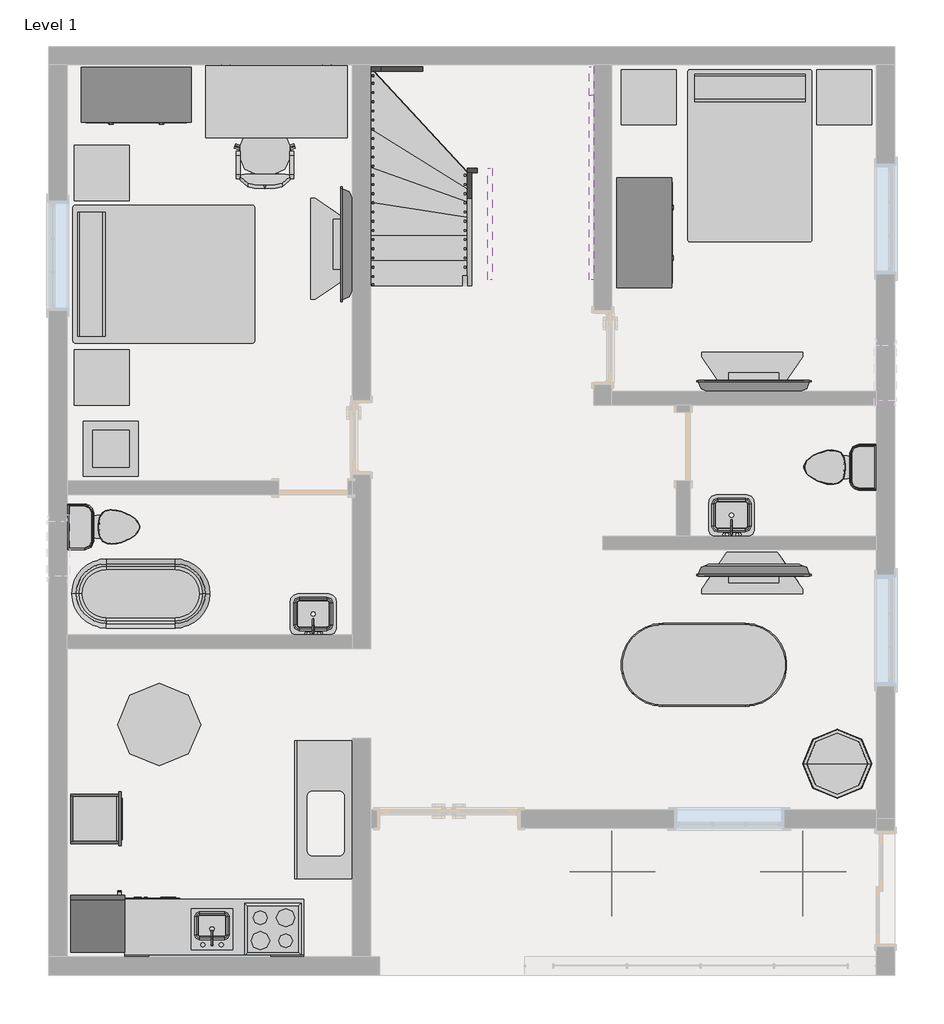
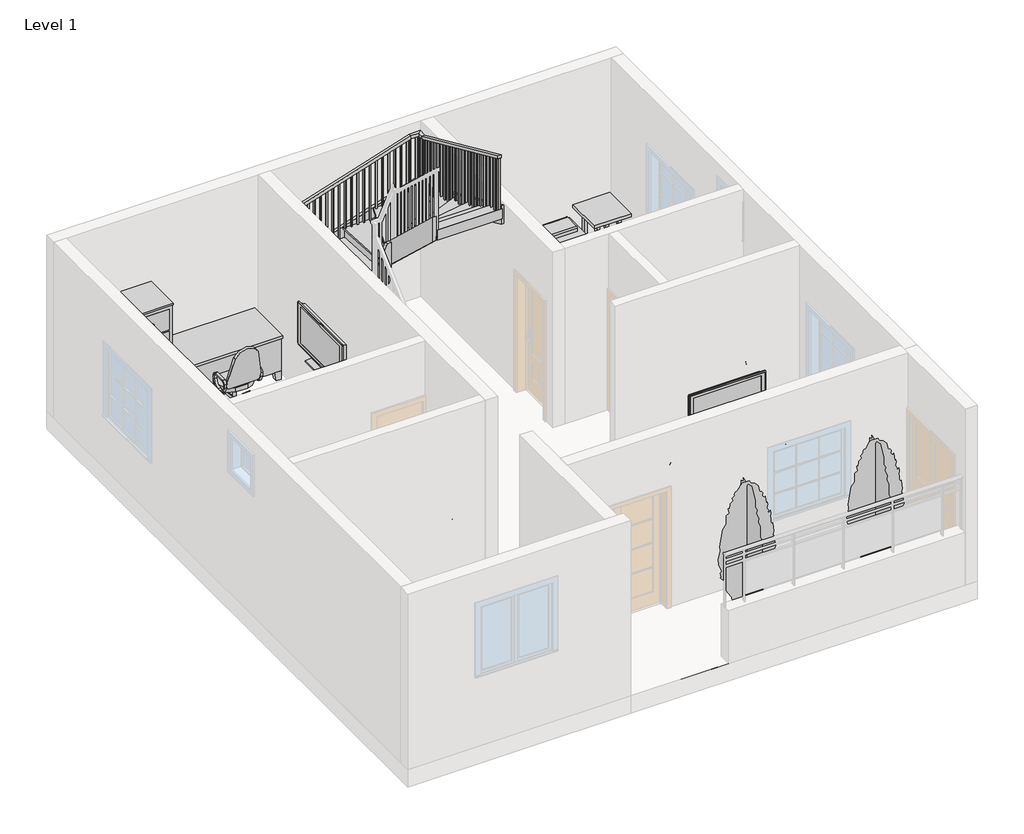
# One storey, part 2 of 2: 22 furniture elements, 8 members, 6 flow terminals, 6 proxies, 2 geographic elements, 1 railing, 1 stair flight.
"""IFC4 building model written with IfcOpenShell, lengths in millimetres."""

from ifc_helpers import new_model, si_unit, frame, origin, place, context, project, spatial, polyline, outline, extrude, faceted_brep, triangles, transform, mapped, element, save
from components import proxy_a6faaae8, proxy_45b28599, kitchenette_medium_kitchenette_medium_844211aa, proxy_8b8c2dc4, proxy_c523a7b7, flow_terminal_871c2e40, flow_terminal_62a433f7, toilet_domestic_3d_toilet_domestic_3d_f7549cf7, toilet_domestic_3d_toilet_domestic_3d_183bbd19, flow_terminal_b374fae2, furniture_0253826f, furniture_e1791683, chair_executive_chair_executive_8d69e98c, furniture_c6510c7c, furniture_6430aa70, furniture_072f6425, furniture_9fa109b2, furniture_fdf74506, tv_stand_tv_stand_6ce107e5, furniture_b5c51a22, furniture_2c34a4f9, furniture_905aceb5, furniture_5bc9ed15, furniture_ebfaaaa6, rpc_tree_conifer_chinese_juniper_7_1b9786cd, stair_flight_3064df67

model = new_model("IFC4")

# Units and contexts
model_context = context("Model", 3, world=origin())
ifc_project = project(units=[si_unit("LENGTHUNIT", "METRE", prefix="MILLI")], contexts=[model_context])

# Site, building, storey
site = spatial("IfcSite", under=ifc_project)
building = spatial("IfcBuilding", under=site)
storey = spatial("IfcBuildingStorey", under=building, Name="Level 1", Elevation=0.0)

# Proxies
placement = place(None, origin())
element("IfcBuildingElementProxy", 1, Name="Building Element Proxy", at=placement, inside=storey, context=model_context, shape_type="Tessellation", body=[
    triangles([(-8321.547876, 2776.9674156, 0.0), (-8317.1533768, 1400.6475002, 0.0), (-8215.9921097, 1395.5161274, 0.0), (-8214.5265015, 1174.0855299, 0.0), (-6665.8942841, 1174.0855299, 0.0), (-6657.047731, 1395.5938843, 0.0), (-6691.0613525, 2780.6355057, 0.0), (-2754.0612556, 2761.5855057, 0.0), (-2754.0612556, 1377.2855541, 0.0)], [[3, 4, 5], [4, 3, 2], [1, 2, 3], [3, 7, 1], [5, 9, 6], [7, 6, 8], [7, 3, 6], [8, 6, 9], [6, 3, 5]], closed=False),
])
proxy_shape = proxy_a6faaae8(model_context)
element("IfcBuildingElementProxy", 2, Name="Cook Top-4 Unit2 : 22\" x 20\"", ObjectType="Cook Top-4 Unit2 : 22\" x 20\"", at=placement, inside=storey, context=model_context, shape_type="MappedRepresentation", body=[
    mapped(proxy_shape, transform((-9421.5611447, 1682.085558, 0.0), x_axis=(-1.0000000000000004, 0.0, 0.0), y_axis=(0.0, -1.0000000000000004, 0.0), z_axis=(0.0, 0.0, 1.0))),
])
proxy_2_shape = proxy_45b28599(model_context)
element("IfcBuildingElementProxy", 3, Name="Dishwasher : 24\" x 24\" x 34\"", ObjectType="Dishwasher : 24\" x 24\" x 34\"", at=placement, inside=storey, context=model_context, shape_type="MappedRepresentation", body=[
    mapped(proxy_2_shape, transform((-10372.7436762, 1973.9351228, 0.0), x_axis=(-1.0000000000000004, 0.0, 0.0), y_axis=(0.0, -1.0000000000000004, 0.0), z_axis=(0.0, 0.0, 1.0))),
])
kitchenette_medium_kitchenette_medium_shape = kitchenette_medium_kitchenette_medium_844211aa(model_context)
element("IfcBuildingElementProxy", 4, Name="Kitchenette - Medium : Kitchenette - Medium", ObjectType="Kitchenette - Medium : Kitchenette - Medium", at=placement, inside=storey, context=model_context, shape_type="MappedRepresentation", body=[
    mapped(kitchenette_medium_kitchenette_medium_shape, transform((-9745.7234398, 1377.285558, 0.0), x_axis=(-1.0000000000000004, 0.0, 0.0), y_axis=(0.0, -1.0000000000000004, 0.0), z_axis=(0.0, 0.0, 1.0))),
])
proxy_3_shape = proxy_8b8c2dc4(model_context)
element("IfcBuildingElementProxy", 5, Name="Oven Double-Built-in : 21 1/2\" x 39 1/4\" x 21\"", ObjectType="Oven Double-Built-in : 21 1/2\" x 39 1/4\" x 21\"", at=placement, inside=storey, context=model_context, shape_type="MappedRepresentation", body=[
    mapped(proxy_3_shape, transform((-11248.9952858, 2936.4604853, 0.0), x_axis=(0.0, 1.0000000000000002, 0.0), y_axis=(-1.0000000000000002, 0.0, 0.0), z_axis=(0.0, 0.0, 1.0))),
])
proxy_4_shape = proxy_c523a7b7(model_context)
element("IfcBuildingElementProxy", 6, Name="Refrigerator : 24\" x 25\" LH", ObjectType="Refrigerator : 24\" x 25\" LH", at=placement, inside=storey, context=model_context, shape_type="MappedRepresentation", body=[
    mapped(proxy_4_shape, transform((-11358.3111447, 1727.7345295, 0.0), x_axis=(-1.0000000000000004, 0.0, 0.0), y_axis=(0.0, -1.0000000000000004, 0.0), z_axis=(0.0, 0.0, 1.0))),
])

# Flow terminals
flow_terminal_shape = flow_terminal_871c2e40(model_context)
element("IfcFlowTerminal", 7, ObjectType="Sink Kitchen-Island : 18\" x 18\"", at=placement, inside=storey, context=model_context, shape_type="MappedRepresentation", body=[
    mapped(flow_terminal_shape, transform((-10078.9719042, 1684.4309591, -14.4), x_axis=(-1.0000000000000004, 0.0, 0.0), y_axis=(0.0, -1.0000000000000004, 0.0), z_axis=(0.0, 0.0, 1.0))),
])
flow_terminal_2_shape = flow_terminal_62a433f7(model_context)
element("IfcFlowTerminal", 8, ObjectType="Sink Vanity-Square : 20\" x 18\"", at=placement, inside=storey, context=model_context, shape_type="MappedRepresentation", body=[
    mapped(flow_terminal_2_shape, transform((-8961.3719042, 5113.4309591, 0.0), x_axis=(-0.9999999999999998, 0.0, 0.0), y_axis=(0.0, -0.9999999999999998, 0.0), z_axis=(0.0, 0.0, 1.0))),
])
element("IfcFlowTerminal", 9, ObjectType="Sink Vanity-Square : 20\" x 18\"", at=placement, inside=storey, context=model_context, shape_type="MappedRepresentation", body=[
    mapped(flow_terminal_2_shape, transform((-4338.5719042, 6205.6309591, 0.0), x_axis=(-1.0, 0.0, 0.0), y_axis=(0.0, -1.0, 0.0), z_axis=(0.0, 0.0, 1.0))),
])
toilet_domestic_3d_toilet_domestic_3d_shape = toilet_domestic_3d_toilet_domestic_3d_f7549cf7(model_context)
toilet_domestic_3d_toilet_domestic_3d_2_shape = toilet_domestic_3d_toilet_domestic_3d_183bbd19(model_context)
element("IfcFlowTerminal", 10, ObjectType="Toilet-Domestic-3D : Toilet-Domestic-3D", at=placement, inside=storey, context=model_context, shape_type="MappedRepresentation", body=[
    mapped(toilet_domestic_3d_toilet_domestic_3d_shape, transform((-11200.1651174, 6127.085558, 0.0), x_axis=(0.0, 1.0000000000000002, 0.0), y_axis=(-1.0000000000000002, 0.0, 0.0), z_axis=(0.0, 0.0, 1.0))),
    mapped(toilet_domestic_3d_toilet_domestic_3d_2_shape, transform((-11200.1651174, 6127.085558, 0.0), x_axis=(0.0, 1.0000000000000002, 0.0), y_axis=(-1.0000000000000002, 0.0, 0.0), z_axis=(0.0, 0.0, 1.0))),
])
element("IfcFlowTerminal", 11, ObjectType="Toilet-Domestic-3D : Toilet-Domestic-3D", at=placement, inside=storey, context=model_context, shape_type="MappedRepresentation", body=[
    mapped(toilet_domestic_3d_toilet_domestic_3d_shape, transform((-3248.7571721, 6787.485558, 0.0), x_axis=(0.0, -1.0000000000000002, 0.0), y_axis=(1.0000000000000002, 0.0, 0.0), z_axis=(0.0, 0.0, 1.0))),
    mapped(toilet_domestic_3d_toilet_domestic_3d_2_shape, transform((-3248.7571721, 6787.485558, 0.0), x_axis=(0.0, -1.0000000000000002, 0.0), y_axis=(1.0000000000000002, 0.0, 0.0), z_axis=(0.0, 0.0, 1.0))),
])
flow_terminal_3_shape = flow_terminal_b374fae2(model_context)
element("IfcFlowTerminal", 12, ObjectType="Tub-Free Standing-3D : 30\" x 60\"", at=placement, inside=storey, context=model_context, shape_type="MappedRepresentation", body=[
    mapped(flow_terminal_3_shape, transform((-10882.0611447, 5390.485558, 0.0), x_axis=(0.0, 1.0, 0.0), y_axis=(-1.0, 0.0, 0.0), z_axis=(0.0, 0.0, 1.0))),
])

# Furniture
furniture_shape = furniture_0253826f(model_context)
element("IfcFurniture", 13, ObjectType="Bed-Standard.0001 : Double 54\" x 75\"", at=placement, inside=storey, context=model_context, shape_type="MappedRepresentation", body=[
    mapped(furniture_shape, transform((-4422.5496693, 10274.78064, 0.0), x_axis=(1.0, 0.0, 0.0), y_axis=(0.0, 1.0, 0.0), z_axis=(0.0, 0.0, 1.0))),
])
furniture_2_shape = furniture_e1791683(model_context)
element("IfcFurniture", 14, ObjectType="Bed-Standard.0001 : Queen 60\" x 79\"", at=placement, inside=storey, context=model_context, shape_type="MappedRepresentation", body=[
    mapped(furniture_2_shape, transform((-10673.6562267, 8649.5970334, 0.0), x_axis=(0.0, 1.0, 0.0), y_axis=(-1.0, 0.0, 0.0), z_axis=(0.0, 0.0, 1.0))),
])
chair_executive_chair_executive_shape = chair_executive_chair_executive_8d69e98c(model_context)
element("IfcFurniture", 15, ObjectType="Chair-Executive : Chair-Executive", at=placement, inside=storey, context=model_context, shape_type="MappedRepresentation", body=[
    mapped(chair_executive_chair_executive_shape, transform((-9651.4519644, 10210.2396563, 0.0), x_axis=(1.0, 0.0, 0.0), y_axis=(0.0, 1.0, 0.0), z_axis=(0.0, 0.0, 1.0))),
])
furniture_3_shape = furniture_c6510c7c(model_context)
element("IfcFurniture", 16, ObjectType="Counter Top w Sink Hole : 24\" Depth", at=placement, inside=storey, context=model_context, shape_type="MappedRepresentation", body=[
    mapped(furniture_3_shape, transform((-10279.1234398, 1377.285558, -14.4), x_axis=(-1.0000000000000004, 0.0, 0.0), y_axis=(0.0, -1.0000000000000004, 0.0), z_axis=(0.0, 0.0, 1.0))),
])
furniture_4_shape = furniture_6430aa70(model_context)
element("IfcFurniture", 17, ObjectType="Counter Top w Sink Hole : 24\" Depth", at=placement, inside=storey, context=model_context, shape_type="MappedRepresentation", body=[
    mapped(furniture_4_shape, transform((-9180.2611447, 3441.3478531, 0.0), x_axis=(0.0, 1.0000000000000002, 0.0), y_axis=(-1.0000000000000002, 0.0, 0.0), z_axis=(0.0, 0.0, 1.0))),
])
furniture_5_shape = furniture_072f6425(model_context)
element("IfcFurniture", 18, ObjectType="Desk : 60\" x 30\"", at=placement, inside=storey, context=model_context, shape_type="MappedRepresentation", body=[
    mapped(furniture_5_shape, transform((-10145.4611447, 10445.085558, 0.0), x_axis=(1.0, 0.0, 0.0), y_axis=(0.0, 1.0, 0.0), z_axis=(0.0, 0.0, 1.0))),
])
furniture_6_shape = furniture_9fa109b2(model_context)
element("IfcFurniture", 19, ObjectType="Dresser : 48\" x 72\" x 24\"", at=placement, inside=storey, context=model_context, shape_type="MappedRepresentation", body=[
    mapped(furniture_6_shape, transform((-10663.6678849, 11265.4485121, 0.0), x_axis=(1.0, 0.0, 0.0), y_axis=(0.0, 1.0, 0.0), z_axis=(0.0, 0.0, 1.0))),
])
element("IfcFurniture", 20, ObjectType="Dresser : 48\" x 72\" x 24\"", at=placement, inside=storey, context=model_context, shape_type="MappedRepresentation", body=[
    mapped(furniture_6_shape, transform((-5682.6240988, 9647.4788178, 0.0), x_axis=(0.0, 1.0, 0.0), y_axis=(-1.0, 0.0, 0.0), z_axis=(0.0, 0.0, 1.0))),
])
furniture_7_shape = furniture_fdf74506(model_context)
element("IfcFurniture", 21, ObjectType="TV - Flat Screen : 50\"", at=placement, inside=storey, context=model_context, shape_type="MappedRepresentation", body=[
    mapped(furniture_7_shape, transform((-8603.7997684, 9247.3410438, 914.4), x_axis=(0.0, -1.0, 0.0), y_axis=(1.0, 0.0, 0.0), z_axis=(0.0, 0.0, 1.0))),
])
element("IfcFurniture", 22, ObjectType="TV - Flat Screen : 50\"", at=placement, inside=storey, context=model_context, shape_type="MappedRepresentation", body=[
    mapped(furniture_7_shape, transform((-4110.5556589, 7677.8741816, 914.4), x_axis=(-1.0, 0.0, 0.0), y_axis=(0.0, -1.0, 0.0), z_axis=(0.0, 0.0, 1.0))),
])
element("IfcFurniture", 23, ObjectType="TV - Flat Screen : 50\"", at=placement, inside=storey, context=model_context, shape_type="MappedRepresentation", body=[
    mapped(furniture_7_shape, transform((-4102.6666306, 5653.9369555, 495.3), x_axis=(1.0, 0.0, 0.0), y_axis=(0.0, 1.0, 0.0), z_axis=(0.0, 0.0, 1.0))),
])
tv_stand_tv_stand_shape = tv_stand_tv_stand_6ce107e5(model_context)
element("IfcFurniture", 24, ObjectType="TV Stand : TV Stand", at=placement, inside=storey, context=model_context, shape_type="MappedRepresentation", body=[
    mapped(tv_stand_tv_stand_shape, transform((-8545.2611447, 9325.6735601, 0.0), x_axis=(0.0, -1.0000000000000002, 0.0), y_axis=(1.0000000000000002, 0.0, 0.0), z_axis=(0.0, 0.0, 1.0))),
])
element("IfcFurniture", 25, ObjectType="TV Stand : TV Stand", at=placement, inside=storey, context=model_context, shape_type="MappedRepresentation", body=[
    mapped(tv_stand_tv_stand_shape, transform((-4000.4731427, 7600.285558, 0.0), x_axis=(-1.0000000000000002, 0.0, 0.0), y_axis=(0.0, -1.0000000000000002, 0.0), z_axis=(0.0, 0.0, 1.0))),
])
element("IfcFurniture", 26, ObjectType="TV Stand : TV Stand", at=placement, inside=storey, context=model_context, shape_type="MappedRepresentation", body=[
    mapped(tv_stand_tv_stand_shape, transform((-4250.8491468, 5847.685558, 0.0), x_axis=(1.0, 0.0, 0.0), y_axis=(0.0, 1.0, 0.0), z_axis=(0.0, 0.0, 1.0))),
])
furniture_8_shape = furniture_b5c51a22(model_context)
element("IfcFurniture", 27, ObjectType="Table-Coffee : 24\" x 24\" x 24\"", at=placement, inside=storey, context=model_context, shape_type="MappedRepresentation", body=[
    mapped(furniture_8_shape, transform((-11230.5269114, 6895.4744802, 0.0), x_axis=(1.0, 0.0, 0.0), y_axis=(0.0, 1.0, 0.0), z_axis=(0.0, 0.0, 1.0))),
])
furniture_9_shape = furniture_2c34a4f9(model_context)
element("IfcFurniture", 28, ObjectType="Table-Dining Oval : 36\" x 72\"", at=placement, inside=storey, context=model_context, shape_type="MappedRepresentation", body=[
    mapped(furniture_9_shape, transform((-4257.2414726, 4961.1839186, 0.0), x_axis=(1.0, 0.0, 0.0), y_axis=(0.0, 1.0, 0.0), z_axis=(0.0, 0.0, 1.0))),
])
furniture_10_shape = furniture_905aceb5(model_context)
element("IfcFurniture", 29, ObjectType="Table-Dining Round w Chairs : 36\" Diameter", at=placement, inside=storey, context=model_context, shape_type="MappedRepresentation", body=[
    mapped(furniture_10_shape, transform((-10782.5431119, 4127.5642465, 0.0), x_axis=(1.0, 0.0, 0.0), y_axis=(0.0, 1.0, 0.0), z_axis=(0.0, 0.0, 1.0))),
])
furniture_11_shape = furniture_5bc9ed15(model_context)
element("IfcFurniture", 30, ObjectType="Table-Night Stand : 24\" x 24\" x 30\"", at=placement, inside=storey, context=model_context, shape_type="MappedRepresentation", body=[
    mapped(furniture_11_shape, transform((-3418.194775, 10572.085558, 0.0), x_axis=(1.0, 0.0, 0.0), y_axis=(0.0, 1.0, 0.0), z_axis=(0.0, 0.0, 1.0))),
])
element("IfcFurniture", 31, ObjectType="Table-Night Stand : 24\" x 24\" x 30\"", at=placement, inside=storey, context=model_context, shape_type="MappedRepresentation", body=[
    mapped(furniture_11_shape, transform((-5577.194775, 10572.085558, 0.0), x_axis=(1.0, 0.0, 0.0), y_axis=(0.0, 1.0, 0.0), z_axis=(0.0, 0.0, 1.0))),
])
element("IfcFurniture", 32, ObjectType="Table-Night Stand : 24\" x 24\" x 30\"", at=placement, inside=storey, context=model_context, shape_type="MappedRepresentation", body=[
    mapped(furniture_11_shape, transform((-11622.394775, 7473.285558, 0.0), x_axis=(1.0, 0.0, 0.0), y_axis=(0.0, 1.0, 0.0), z_axis=(0.0, 0.0, 1.0))),
])
element("IfcFurniture", 33, ObjectType="Table-Night Stand : 24\" x 24\" x 30\"", at=placement, inside=storey, context=model_context, shape_type="MappedRepresentation", body=[
    mapped(furniture_11_shape, transform((-11622.394775, 9733.885558, 0.0), x_axis=(1.0, 0.0, 0.0), y_axis=(0.0, 1.0, 0.0), z_axis=(0.0, 0.0, 1.0))),
])
furniture_12_shape = furniture_ebfaaaa6(model_context)
element("IfcFurniture", 34, ObjectType="Table-Round : 36\" Diameter", at=placement, inside=storey, context=model_context, shape_type="MappedRepresentation", body=[
    mapped(furniture_12_shape, transform((-3185.8611447, 3510.885558, 0.0), x_axis=(1.0, 0.0, 0.0), y_axis=(0.0, 1.0, 0.0), z_axis=(0.0, 0.0, 1.0))),
])

# Geographic elements
rpc_tree_conifer_chinese_juniper_7_shape = rpc_tree_conifer_chinese_juniper_7_1b9786cd(model_context)
element("IfcGeographicElement", 35, ObjectType="RPC Tree - Conifer : Chinese Juniper - 7'", at=placement, inside=storey, context=model_context, shape_type="MappedRepresentation", body=[
    mapped(rpc_tree_conifer_chinese_juniper_7_shape, transform((-5675.2578158, 2317.085558, 0.0), x_axis=(1.0, 0.0, 0.0), y_axis=(0.0, 1.0, 0.0), z_axis=(0.0, 0.0, 1.0))),
])
element("IfcGeographicElement", 36, ObjectType="RPC Tree - Conifer : Chinese Juniper - 7'", at=placement, inside=storey, context=model_context, shape_type="MappedRepresentation", body=[
    mapped(rpc_tree_conifer_chinese_juniper_7_shape, transform((-3567.0578158, 2317.085558, 0.0), x_axis=(1.0, 0.0, 0.0), y_axis=(0.0, 1.0, 0.0), z_axis=(0.0, 0.0, 1.0))),
])

# Members
element("IfcMember", 37, ObjectType="Stringer - 2\" Width", at=placement, inside=storey, context=model_context, shape_type="SweptSolid", body=[
    extrude(outline(polyline([(8794.085558, 93.014189), (8794.085558, 421.9745329), (11160.0172498, 1382.4832821), (11160.0172498, 1053.5229382), (8794.085558, 93.014189)])), frame((-8392.8611447, 0.0, 0.0), z_axis=(1.0, 0.0, 0.0), x_axis=(0.0, 1.0, 0.0)), (0.0, 0.0, 1.0), 50.8),
])
element("IfcMember", 38, ObjectType="Stringer - 2\" Width", at=placement, inside=storey, context=model_context, shape_type="SweptSolid", body=[
    extrude(outline(polyline([(-8392.8611447, 11160.0172498), (-8392.8611447, 11210.8172498), (-8228.6602308, 11210.8172498), (-8228.6602308, 11160.0172498), (-8392.8611447, 11160.0172498)])), frame((0.0, 0.0, 1053.5229382), z_axis=(0.0, 0.0, 1.0), x_axis=(1.0, 0.0, 0.0)), (0.0, 0.0, 1.0), 328.9603439),
])
element("IfcMember", 39, ObjectType="Stringer - 2\" Width", at=placement, inside=storey, context=model_context, shape_type="SweptSolid", body=[
    extrude(outline(polyline([(1382.4832821, -8228.6602308), (1053.5229382, -8228.6602308), (1784.8447546, -5929.0611447), (2109.3790897, -5929.0611447), (2109.3790897, -5942.9784728), (1382.4832821, -8228.6602308)])), frame((0.0, 11160.0172498, 0.0), z_axis=(0.0, 1.0, 0.0), x_axis=(0.0, 0.0, 1.0)), (0.0, 0.0, 1.0), 50.8),
])
element("IfcMember", 40, ObjectType="Stringer - 2\" Width", at=placement, inside=storey, context=model_context, shape_type="SweptSolid", body=[
    extrude(outline(polyline([(-5929.0611447, 11210.8172498), (-5878.2611447, 11210.8172498), (-5878.2611447, 10897.3150688), (-5929.0611447, 10897.3150688), (-5929.0611447, 11210.8172498)])), frame((0.0, 0.0, 1789.5368881), z_axis=(0.0, 0.0, 1.0), x_axis=(1.0, 0.0, 0.0)), (0.0, 0.0, 1.0), 319.8422017),
])
element("IfcMember", 41, ObjectType="Stringer - 2\" Width", at=placement, inside=storey, context=model_context, shape_type="SweptSolid", body=[
    extrude(outline(polyline([(10897.3150688, 2109.3790897), (10897.3150688, 1789.5368881), (8859.8360051, 2707.7119272), (8859.8360051, 3027.5541288), (10897.3150688, 2109.3790897)])), frame((-5929.0611447, 0.0, 0.0), z_axis=(1.0, 0.0, 0.0), x_axis=(0.0, 1.0, 0.0)), (0.0, 0.0, 1.0), 50.8),
])
element("IfcMember", 42, ObjectType="Stringer - 2\" Width", at=placement, inside=storey, context=model_context, shape_type="SweptSolid", body=[
    extrude(outline(polyline([(8794.085558, 0.0), (8794.085558, 331.5187421), (10042.4172498, 1462.9448948), (10042.4172498, 1051.5810316), (8882.1807419, 0.0), (8794.085558, 0.0)])), frame((-7275.2611447, 0.0, 0.0), z_axis=(1.0, 0.0, 0.0), x_axis=(0.0, 1.0, 0.0)), (0.0, 0.0, 1.0), 50.8),
])
element("IfcMember", 43, ObjectType="Stringer - 2\" Width", at=placement, inside=storey, context=model_context, shape_type="SweptSolid", body=[
    extrude(outline(polyline([(1707.5062782, -7275.2611447), (1097.6236411, -7275.2611447), (1097.6236411, -7209.7683833), (1469.7815899, -7046.6611447), (2069.9469496, -7046.6611447), (2069.9469496, -7116.4127385), (1707.5062782, -7275.2611447)])), frame((0.0, 10042.4172498, 0.0), z_axis=(0.0, 1.0, 0.0), x_axis=(0.0, 0.0, 1.0)), (0.0, 0.0, 1.0), 50.8),
])
element("IfcMember", 44, ObjectType="Stringer - 2\" Width", at=placement, inside=storey, context=model_context, shape_type="SweptSolid", body=[
    extrude(outline(polyline([(10093.2172498, 2069.9469496), (10093.2172498, 1653.3593378), (8859.8360051, 2802.474504), (8859.8360051, 3219.0621158), (10093.2172498, 2069.9469496)])), frame((-7046.6611447, 0.0, 0.0), z_axis=(1.0, 0.0, 0.0), x_axis=(0.0, 1.0, 0.0)), (0.0, 0.0, 1.0), 50.8),
])

# Railing
element("IfcRailing", 45, ObjectType="Handrail - Rectangular", at=placement, inside=storey, context=model_context, shape_type="SolidModel", body=[
    faceted_brep([(-8342.0611447, 8794.085558, 1308.9706286), (-8342.0611447, 8794.085558, 1254.1439046), (-8291.2611447, 8794.085558, 1254.1439046), (-8291.2611447, 8794.085558, 1308.9706286), (-8342.0611447, 11033.0172498, 2217.9205727), (-8342.0611447, 11083.8172498, 2183.7173707), (-8291.2611447, 11083.8172498, 2183.7173707), (-8291.2611447, 11033.0172498, 2217.9205727), (-6102.00887, 11160.0172498, 2892.4930757), (-6109.8920919, 11160.0172498, 2943.2930757), (-5929.0611447, 11160.0172498, 2943.2930757), (-5929.0611447, 11160.0172498, 2892.4930757), (-6102.00887, 11109.2172498, 2892.4930757), (-5979.8611447, 11109.2172498, 2892.4930757), (-6109.8920919, 11109.2172498, 2943.2930757), (-5979.8611447, 11109.2172498, 2943.2930757), (-8207.1779228, 11160.0172498, 2223.0041788), (-8215.0611447, 11160.0172498, 2273.8041788), (-8207.1779228, 11109.2172498, 2223.0041788), (-8215.0611447, 11109.2172498, 2273.8041788), (-5929.0611447, 8859.8360051, 3918.9762333), (-5979.8611447, 8859.8360051, 3918.9762333), (-5979.8611447, 8859.8360051, 3863.2562786), (-5929.0611447, 8859.8360051, 3863.2562786), (-5929.0611447, 11014.0109908, 2892.4930757), (-5929.0611447, 11024.928631, 2943.2930757), (-5979.8611447, 11014.0109908, 2892.4930757), (-5979.8611447, 11024.928631, 2943.2930757), (-8342.0611447, 11033.0172498, 2273.8041788), (-8342.0611447, 11083.8172498, 2223.0041788), (-8291.2611447, 11083.8172498, 2223.0041788), (-8291.2611447, 11033.0172498, 2273.8041788), (-8342.0611447, 11160.0172498, 2273.8041788), (-8342.0611447, 11160.0172498, 2223.0041788), (-8291.2611447, 11109.2172498, 2223.0041788), (-8291.2611447, 11109.2172498, 2273.8041788)], [[[0, 1, 2, 3]], [[1, 0, 4, 5]], [[2, 1, 5, 6]], [[3, 2, 6, 7]], [[0, 3, 7, 4]], [[8, 9, 10, 11]], [[12, 8, 11, 13]], [[14, 12, 13, 15]], [[9, 14, 15, 10]], [[16, 17, 9, 8]], [[18, 16, 8, 12]], [[19, 18, 12, 14]], [[17, 19, 14, 9]], [[20, 21, 22, 23]], [[24, 25, 20, 23]], [[26, 24, 23, 22]], [[27, 26, 22, 21]], [[25, 27, 21, 20]], [[11, 10, 25, 24]], [[13, 11, 24, 26]], [[15, 13, 26, 27]], [[10, 15, 27, 25]], [[5, 4, 28, 29]], [[6, 5, 29, 30]], [[7, 6, 30, 31]], [[4, 7, 31, 28]], [[29, 28, 32, 33]], [[30, 29, 33, 34]], [[31, 30, 34, 35]], [[28, 31, 35, 32]], [[33, 32, 17, 16]], [[34, 33, 16, 18]], [[35, 34, 18, 19]], [[32, 35, 19, 17]]]),
    extrude(outline(polyline([(8900.853631, 3844.7719855), (8900.853631, 2878.6666667), (8881.803631, 2878.6666667), (8881.803631, 3853.3567286), (8900.853631, 3844.7719855)])), frame((-5963.9861447, 0.0, 0.0), z_axis=(1.0, 0.0, 0.0), x_axis=(0.0, 1.0, 0.0)), (0.0, 0.0, 1.0), 19.05),
    extrude(outline(polyline([(9002.453631, 3798.9866885), (9002.453631, 2878.6666667), (8983.403631, 2878.6666667), (8983.403631, 3807.5714317), (9002.453631, 3798.9866885)])), frame((-5963.9861447, 0.0, 0.0), z_axis=(1.0, 0.0, 0.0), x_axis=(0.0, 1.0, 0.0)), (0.0, 0.0, 1.0), 19.05),
    extrude(outline(polyline([(9104.053631, 3753.2013916), (9104.053631, 2878.6666667), (9085.003631, 2878.6666667), (9085.003631, 3761.7861347), (9104.053631, 3753.2013916)])), frame((-5963.9861447, 0.0, 0.0), z_axis=(1.0, 0.0, 0.0), x_axis=(0.0, 1.0, 0.0)), (0.0, 0.0, 1.0), 19.05),
    extrude(outline(polyline([(9205.653631, 3707.4160946), (9205.653631, 2709.3333333), (9186.603631, 2709.3333333), (9186.603631, 3716.0008378), (9205.653631, 3707.4160946)])), frame((-5963.9861447, 0.0, 0.0), z_axis=(1.0, 0.0, 0.0), x_axis=(0.0, 1.0, 0.0)), (0.0, 0.0, 1.0), 19.05),
    extrude(outline(polyline([(9307.253631, 3661.6307976), (9307.253631, 2709.3333333), (9288.203631, 2709.3333333), (9288.203631, 3670.2155408), (9307.253631, 3661.6307976)])), frame((-5963.9861447, 0.0, 0.0), z_axis=(1.0, 0.0, 0.0), x_axis=(0.0, 1.0, 0.0)), (0.0, 0.0, 1.0), 19.05),
    extrude(outline(polyline([(9408.853631, 3615.8455007), (9408.853631, 2709.3333333), (9389.803631, 2709.3333333), (9389.803631, 3624.4302439), (9408.853631, 3615.8455007)])), frame((-5963.9861447, 0.0, 0.0), z_axis=(1.0, 0.0, 0.0), x_axis=(0.0, 1.0, 0.0)), (0.0, 0.0, 1.0), 19.05),
    extrude(outline(polyline([(9510.453631, 3570.0602037), (9510.453631, 2540.0), (9491.403631, 2540.0), (9491.403631, 3578.6449469), (9510.453631, 3570.0602037)])), frame((-5963.9861447, 0.0, 0.0), z_axis=(1.0, 0.0, 0.0), x_axis=(0.0, 1.0, 0.0)), (0.0, 0.0, 1.0), 19.05),
    extrude(outline(polyline([(9612.053631, 3524.2749068), (9612.053631, 2540.0), (9593.003631, 2540.0), (9593.003631, 3532.85965), (9612.053631, 3524.2749068)])), frame((-5963.9861447, 0.0, 0.0), z_axis=(1.0, 0.0, 0.0), x_axis=(0.0, 1.0, 0.0)), (0.0, 0.0, 1.0), 19.05),
    extrude(outline(polyline([(9713.653631, 3478.4896098), (9713.653631, 2540.0), (9694.603631, 2540.0), (9694.603631, 3487.074353), (9713.653631, 3478.4896098)])), frame((-5963.9861447, 0.0, 0.0), z_axis=(1.0, 0.0, 0.0), x_axis=(0.0, 1.0, 0.0)), (0.0, 0.0, 1.0), 19.05),
    extrude(outline(polyline([(9815.253631, 3432.7043129), (9815.253631, 2370.6666667), (9796.203631, 2370.6666667), (9796.203631, 3441.289056), (9815.253631, 3432.7043129)])), frame((-5963.9861447, 0.0, 0.0), z_axis=(1.0, 0.0, 0.0), x_axis=(0.0, 1.0, 0.0)), (0.0, 0.0, 1.0), 19.05),
    extrude(outline(polyline([(9916.853631, 3386.9190159), (9916.853631, 2370.6666667), (9897.803631, 2370.6666667), (9897.803631, 3395.5037591), (9916.853631, 3386.9190159)])), frame((-5963.9861447, 0.0, 0.0), z_axis=(1.0, 0.0, 0.0), x_axis=(0.0, 1.0, 0.0)), (0.0, 0.0, 1.0), 19.05),
    extrude(outline(polyline([(10018.453631, 3341.1337189), (10018.453631, 2370.6666667), (9999.403631, 2370.6666667), (9999.403631, 3349.7184621), (10018.453631, 3341.1337189)])), frame((-5963.9861447, 0.0, 0.0), z_axis=(1.0, 0.0, 0.0), x_axis=(0.0, 1.0, 0.0)), (0.0, 0.0, 1.0), 19.05),
    extrude(outline(polyline([(10120.053631, 3295.348422), (10120.053631, 2370.6666667), (10101.003631, 2370.6666667), (10101.003631, 3303.9331652), (10120.053631, 3295.348422)])), frame((-5963.9861447, 0.0, 0.0), z_axis=(1.0, 0.0, 0.0), x_axis=(0.0, 1.0, 0.0)), (0.0, 0.0, 1.0), 19.05),
    extrude(outline(polyline([(10221.653631, 3249.563125), (10221.653631, 2201.3333333), (10202.603631, 2201.3333333), (10202.603631, 3258.1478682), (10221.653631, 3249.563125)])), frame((-5963.9861447, 0.0, 0.0), z_axis=(1.0, 0.0, 0.0), x_axis=(0.0, 1.0, 0.0)), (0.0, 0.0, 1.0), 19.05),
    extrude(outline(polyline([(10323.253631, 3203.7778281), (10323.253631, 2201.3333333), (10304.203631, 2201.3333333), (10304.203631, 3212.3625713), (10323.253631, 3203.7778281)])), frame((-5963.9861447, 0.0, 0.0), z_axis=(1.0, 0.0, 0.0), x_axis=(0.0, 1.0, 0.0)), (0.0, 0.0, 1.0), 19.05),
    extrude(outline(polyline([(10424.853631, 3157.9925311), (10424.853631, 2201.3333333), (10405.803631, 2201.3333333), (10405.803631, 3166.5772743), (10424.853631, 3157.9925311)])), frame((-5963.9861447, 0.0, 0.0), z_axis=(1.0, 0.0, 0.0), x_axis=(0.0, 1.0, 0.0)), (0.0, 0.0, 1.0), 19.05),
    extrude(outline(polyline([(10526.453631, 3112.2072342), (10526.453631, 2201.3333333), (10507.403631, 2201.3333333), (10507.403631, 3120.7919773), (10526.453631, 3112.2072342)])), frame((-5963.9861447, 0.0, 0.0), z_axis=(1.0, 0.0, 0.0), x_axis=(0.0, 1.0, 0.0)), (0.0, 0.0, 1.0), 19.05),
    extrude(outline(polyline([(10628.053631, 3066.4219372), (10628.053631, 2201.3333333), (10609.003631, 2201.3333333), (10609.003631, 3075.0066804), (10628.053631, 3066.4219372)])), frame((-5963.9861447, 0.0, 0.0), z_axis=(1.0, 0.0, 0.0), x_axis=(0.0, 1.0, 0.0)), (0.0, 0.0, 1.0), 19.05),
    extrude(outline(polyline([(10729.653631, 3020.6366403), (10729.653631, 2032.0), (10710.603631, 2032.0), (10710.603631, 3029.2213834), (10729.653631, 3020.6366403)])), frame((-5963.9861447, 0.0, 0.0), z_axis=(1.0, 0.0, 0.0), x_axis=(0.0, 1.0, 0.0)), (0.0, 0.0, 1.0), 19.05),
    extrude(outline(polyline([(10831.253631, 2974.8513433), (10831.253631, 2032.0), (10812.203631, 2032.0), (10812.203631, 2983.4360865), (10831.253631, 2974.8513433)])), frame((-5963.9861447, 0.0, 0.0), z_axis=(1.0, 0.0, 0.0), x_axis=(0.0, 1.0, 0.0)), (0.0, 0.0, 1.0), 19.05),
    extrude(outline(polyline([(10932.853631, 2929.0660463), (10932.853631, 2032.0), (10913.803631, 2032.0), (10913.803631, 2937.6507895), (10932.853631, 2929.0660463)])), frame((-5963.9861447, 0.0, 0.0), z_axis=(1.0, 0.0, 0.0), x_axis=(0.0, 1.0, 0.0)), (0.0, 0.0, 1.0), 19.05),
    extrude(outline(polyline([(-5944.9361447, 11042.5422498), (-5944.9361447, 11023.4922498), (-5963.9861447, 11023.4922498), (-5963.9861447, 11042.5422498), (-5944.9361447, 11042.5422498)])), frame((0.0, 0.0, 2032.0), z_axis=(0.0, 0.0, 1.0), x_axis=(1.0, 0.0, 0.0)), (0.0, 0.0, 1.0), 860.4930757),
    extrude(outline(polyline([(-6017.8170919, 11144.1422498), (-5998.7670919, 11144.1422498), (-5998.7670919, 11125.0922498), (-6017.8170919, 11125.0922498), (-6017.8170919, 11144.1422498)])), frame((0.0, 0.0, 2032.0), z_axis=(0.0, 0.0, 1.0), x_axis=(1.0, 0.0, 0.0)), (0.0, 0.0, 1.0), 860.4930757),
    extrude(outline(polyline([(2872.5247684, -6164.7980554), (1862.6666667, -6164.7980554), (1862.6666667, -6145.7480554), (2878.5830769, -6145.7480554), (2872.5247684, -6164.7980554)])), frame((0.0, 11125.0922498, 0.0), z_axis=(0.0, 1.0, 0.0), x_axis=(0.0, 0.0, 1.0)), (0.0, 0.0, 1.0), 19.05),
    extrude(outline(polyline([(2840.21379, -6266.3980554), (1862.6666667, -6266.3980554), (1862.6666667, -6247.3480554), (2846.2720984, -6247.3480554), (2840.21379, -6266.3980554)])), frame((0.0, 11125.0922498, 0.0), z_axis=(0.0, 1.0, 0.0), x_axis=(0.0, 0.0, 1.0)), (0.0, 0.0, 1.0), 19.05),
    extrude(outline(polyline([(2807.9028115, -6367.9980554), (1862.6666667, -6367.9980554), (1862.6666667, -6348.9480554), (2813.96112, -6348.9480554), (2807.9028115, -6367.9980554)])), frame((0.0, 11125.0922498, 0.0), z_axis=(0.0, 1.0, 0.0), x_axis=(0.0, 0.0, 1.0)), (0.0, 0.0, 1.0), 19.05),
    extrude(outline(polyline([(2775.5918331, -6469.5980554), (1862.6666667, -6469.5980554), (1862.6666667, -6450.5480554), (2781.6501415, -6450.5480554), (2775.5918331, -6469.5980554)])), frame((0.0, 11125.0922498, 0.0), z_axis=(0.0, 1.0, 0.0), x_axis=(0.0, 0.0, 1.0)), (0.0, 0.0, 1.0), 19.05),
    extrude(outline(polyline([(2743.2808546, -6571.1980554), (1862.6666667, -6571.1980554), (1862.6666667, -6552.1480554), (2749.339163, -6552.1480554), (2743.2808546, -6571.1980554)])), frame((0.0, 11125.0922498, 0.0), z_axis=(0.0, 1.0, 0.0), x_axis=(0.0, 0.0, 1.0)), (0.0, 0.0, 1.0), 19.05),
    extrude(outline(polyline([(2710.9698761, -6672.7980554), (1862.6666667, -6672.7980554), (1862.6666667, -6653.7480554), (2717.0281846, -6653.7480554), (2710.9698761, -6672.7980554)])), frame((0.0, 11125.0922498, 0.0), z_axis=(0.0, 1.0, 0.0), x_axis=(0.0, 0.0, 1.0)), (0.0, 0.0, 1.0), 19.05),
    extrude(outline(polyline([(2678.6588977, -6774.3980554), (1693.3333333, -6774.3980554), (1693.3333333, -6755.3480554), (2684.7172061, -6755.3480554), (2678.6588977, -6774.3980554)])), frame((0.0, 11125.0922498, 0.0), z_axis=(0.0, 1.0, 0.0), x_axis=(0.0, 0.0, 1.0)), (0.0, 0.0, 1.0), 19.05),
    extrude(outline(polyline([(2646.3479192, -6875.9980554), (1693.3333333, -6875.9980554), (1693.3333333, -6856.9480554), (2652.4062277, -6856.9480554), (2646.3479192, -6875.9980554)])), frame((0.0, 11125.0922498, 0.0), z_axis=(0.0, 1.0, 0.0), x_axis=(0.0, 0.0, 1.0)), (0.0, 0.0, 1.0), 19.05),
    extrude(outline(polyline([(2614.0369407, -6977.5980554), (1693.3333333, -6977.5980554), (1693.3333333, -6958.5480554), (2620.0952492, -6958.5480554), (2614.0369407, -6977.5980554)])), frame((0.0, 11125.0922498, 0.0), z_axis=(0.0, 1.0, 0.0), x_axis=(0.0, 0.0, 1.0)), (0.0, 0.0, 1.0), 19.05),
    extrude(outline(polyline([(2581.7259623, -7079.1980554), (1693.3333333, -7079.1980554), (1693.3333333, -7060.1480554), (2587.7842707, -7060.1480554), (2581.7259623, -7079.1980554)])), frame((0.0, 11125.0922498, 0.0), z_axis=(0.0, 1.0, 0.0), x_axis=(0.0, 0.0, 1.0)), (0.0, 0.0, 1.0), 19.05),
    extrude(outline(polyline([(2549.4149838, -7180.7980554), (1693.3333333, -7180.7980554), (1693.3333333, -7161.7480554), (2555.4732923, -7161.7480554), (2549.4149838, -7180.7980554)])), frame((0.0, 11125.0922498, 0.0), z_axis=(0.0, 1.0, 0.0), x_axis=(0.0, 0.0, 1.0)), (0.0, 0.0, 1.0), 19.05),
    extrude(outline(polyline([(2517.1040054, -7282.3980554), (1524.0, -7282.3980554), (1524.0, -7263.3480554), (2523.1623138, -7263.3480554), (2517.1040054, -7282.3980554)])), frame((0.0, 11125.0922498, 0.0), z_axis=(0.0, 1.0, 0.0), x_axis=(0.0, 0.0, 1.0)), (0.0, 0.0, 1.0), 19.05),
    extrude(outline(polyline([(2484.7930269, -7383.9980554), (1524.0, -7383.9980554), (1524.0, -7364.9480554), (2490.8513354, -7364.9480554), (2484.7930269, -7383.9980554)])), frame((0.0, 11125.0922498, 0.0), z_axis=(0.0, 1.0, 0.0), x_axis=(0.0, 0.0, 1.0)), (0.0, 0.0, 1.0), 19.05),
    extrude(outline(polyline([(2452.4820484, -7485.5980554), (1524.0, -7485.5980554), (1524.0, -7466.5480554), (2458.5403569, -7466.5480554), (2452.4820484, -7485.5980554)])), frame((0.0, 11125.0922498, 0.0), z_axis=(0.0, 1.0, 0.0), x_axis=(0.0, 0.0, 1.0)), (0.0, 0.0, 1.0), 19.05),
    extrude(outline(polyline([(2420.17107, -7587.1980554), (1524.0, -7587.1980554), (1524.0, -7568.1480554), (2426.2293784, -7568.1480554), (2420.17107, -7587.1980554)])), frame((0.0, 11125.0922498, 0.0), z_axis=(0.0, 1.0, 0.0), x_axis=(0.0, 0.0, 1.0)), (0.0, 0.0, 1.0), 19.05),
    extrude(outline(polyline([(2387.8600915, -7688.7980554), (1524.0, -7688.7980554), (1524.0, -7669.7480554), (2393.9184, -7669.7480554), (2387.8600915, -7688.7980554)])), frame((0.0, 11125.0922498, 0.0), z_axis=(0.0, 1.0, 0.0), x_axis=(0.0, 0.0, 1.0)), (0.0, 0.0, 1.0), 19.05),
    extrude(outline(polyline([(2355.549113, -7790.3980554), (1354.6666667, -7790.3980554), (1354.6666667, -7771.3480554), (2361.6074215, -7771.3480554), (2355.549113, -7790.3980554)])), frame((0.0, 11125.0922498, 0.0), z_axis=(0.0, 1.0, 0.0), x_axis=(0.0, 0.0, 1.0)), (0.0, 0.0, 1.0), 19.05),
    extrude(outline(polyline([(2323.2381346, -7891.9980554), (1354.6666667, -7891.9980554), (1354.6666667, -7872.9480554), (2329.296443, -7872.9480554), (2323.2381346, -7891.9980554)])), frame((0.0, 11125.0922498, 0.0), z_axis=(0.0, 1.0, 0.0), x_axis=(0.0, 0.0, 1.0)), (0.0, 0.0, 1.0), 19.05),
    extrude(outline(polyline([(2290.9271561, -7993.5980554), (1354.6666667, -7993.5980554), (1354.6666667, -7974.5480554), (2296.9854646, -7974.5480554), (2290.9271561, -7993.5980554)])), frame((0.0, 11125.0922498, 0.0), z_axis=(0.0, 1.0, 0.0), x_axis=(0.0, 0.0, 1.0)), (0.0, 0.0, 1.0), 19.05),
    extrude(outline(polyline([(2258.6161777, -8095.1980554), (1354.6666667, -8095.1980554), (1354.6666667, -8076.1480554), (2264.6744861, -8076.1480554), (2258.6161777, -8095.1980554)])), frame((0.0, 11125.0922498, 0.0), z_axis=(0.0, 1.0, 0.0), x_axis=(0.0, 0.0, 1.0)), (0.0, 0.0, 1.0), 19.05),
    extrude(outline(polyline([(2226.3051992, -8196.7980554), (1354.6666667, -8196.7980554), (1354.6666667, -8177.7480554), (2232.3635077, -8177.7480554), (2226.3051992, -8196.7980554)])), frame((0.0, 11125.0922498, 0.0), z_axis=(0.0, 1.0, 0.0), x_axis=(0.0, 0.0, 1.0)), (0.0, 0.0, 1.0), 19.05),
    extrude(outline(polyline([(11038.810558, 2165.445786), (11038.810558, 1185.3333333), (11019.760558, 1185.3333333), (11019.760558, 2157.7119653), (11038.810558, 2165.445786)])), frame((-8326.1861447, 0.0, 0.0), z_axis=(1.0, 0.0, 0.0), x_axis=(0.0, 1.0, 0.0)), (0.0, 0.0, 1.0), 19.05),
    extrude(outline(polyline([(10937.210558, 2124.1987419), (10937.210558, 1185.3333333), (10918.160558, 1185.3333333), (10918.160558, 2116.4649211), (10937.210558, 2124.1987419)])), frame((-8326.1861447, 0.0, 0.0), z_axis=(1.0, 0.0, 0.0), x_axis=(0.0, 1.0, 0.0)), (0.0, 0.0, 1.0), 19.05),
    extrude(outline(polyline([(10835.610558, 2082.9516978), (10835.610558, 1185.3333333), (10816.560558, 1185.3333333), (10816.560558, 2075.217877), (10835.610558, 2082.9516978)])), frame((-8326.1861447, 0.0, 0.0), z_axis=(1.0, 0.0, 0.0), x_axis=(0.0, 1.0, 0.0)), (0.0, 0.0, 1.0), 19.05),
    extrude(outline(polyline([(10734.010558, 2041.7046536), (10734.010558, 1185.3333333), (10714.960558, 1185.3333333), (10714.960558, 2033.9708329), (10734.010558, 2041.7046536)])), frame((-8326.1861447, 0.0, 0.0), z_axis=(1.0, 0.0, 0.0), x_axis=(0.0, 1.0, 0.0)), (0.0, 0.0, 1.0), 19.05),
    extrude(outline(polyline([(10632.410558, 2000.4576095), (10632.410558, 1185.3333333), (10613.360558, 1185.3333333), (10613.360558, 1992.7237887), (10632.410558, 2000.4576095)])), frame((-8326.1861447, 0.0, 0.0), z_axis=(1.0, 0.0, 0.0), x_axis=(0.0, 1.0, 0.0)), (0.0, 0.0, 1.0), 19.05),
    extrude(outline(polyline([(10530.810558, 1959.2105654), (10530.810558, 1185.3333333), (10511.760558, 1185.3333333), (10511.760558, 1951.4767446), (10530.810558, 1959.2105654)])), frame((-8326.1861447, 0.0, 0.0), z_axis=(1.0, 0.0, 0.0), x_axis=(0.0, 1.0, 0.0)), (0.0, 0.0, 1.0), 19.05),
    extrude(outline(polyline([(10429.210558, 1917.9635212), (10429.210558, 1016.0), (10410.160558, 1016.0), (10410.160558, 1910.2297004), (10429.210558, 1917.9635212)])), frame((-8326.1861447, 0.0, 0.0), z_axis=(1.0, 0.0, 0.0), x_axis=(0.0, 1.0, 0.0)), (0.0, 0.0, 1.0), 19.05),
    extrude(outline(polyline([(10327.610558, 1876.7164771), (10327.610558, 1016.0), (10308.560558, 1016.0), (10308.560558, 1868.9826563), (10327.610558, 1876.7164771)])), frame((-8326.1861447, 0.0, 0.0), z_axis=(1.0, 0.0, 0.0), x_axis=(0.0, 1.0, 0.0)), (0.0, 0.0, 1.0), 19.05),
    extrude(outline(polyline([(10226.010558, 1835.4694329), (10226.010558, 1016.0), (10206.960558, 1016.0), (10206.960558, 1827.7356122), (10226.010558, 1835.4694329)])), frame((-8326.1861447, 0.0, 0.0), z_axis=(1.0, 0.0, 0.0), x_axis=(0.0, 1.0, 0.0)), (0.0, 0.0, 1.0), 19.05),
    extrude(outline(polyline([(10124.410558, 1794.2223888), (10124.410558, 1016.0), (10105.360558, 1016.0), (10105.360558, 1786.488568), (10124.410558, 1794.2223888)])), frame((-8326.1861447, 0.0, 0.0), z_axis=(1.0, 0.0, 0.0), x_axis=(0.0, 1.0, 0.0)), (0.0, 0.0, 1.0), 19.05),
    extrude(outline(polyline([(10022.810558, 1752.9753447), (10022.810558, 846.6666667), (10003.760558, 846.6666667), (10003.760558, 1745.2415239), (10022.810558, 1752.9753447)])), frame((-8326.1861447, 0.0, 0.0), z_axis=(1.0, 0.0, 0.0), x_axis=(0.0, 1.0, 0.0)), (0.0, 0.0, 1.0), 19.05),
    extrude(outline(polyline([(9921.210558, 1711.7283005), (9921.210558, 846.6666667), (9902.160558, 846.6666667), (9902.160558, 1703.9944798), (9921.210558, 1711.7283005)])), frame((-8326.1861447, 0.0, 0.0), z_axis=(1.0, 0.0, 0.0), x_axis=(0.0, 1.0, 0.0)), (0.0, 0.0, 1.0), 19.05),
    extrude(outline(polyline([(9819.610558, 1670.4812564), (9819.610558, 846.6666667), (9800.560558, 846.6666667), (9800.560558, 1662.7474356), (9819.610558, 1670.4812564)])), frame((-8326.1861447, 0.0, 0.0), z_axis=(1.0, 0.0, 0.0), x_axis=(0.0, 1.0, 0.0)), (0.0, 0.0, 1.0), 19.05),
    extrude(outline(polyline([(9718.010558, 1629.2342123), (9718.010558, 677.3333333), (9698.960558, 677.3333333), (9698.960558, 1621.5003915), (9718.010558, 1629.2342123)])), frame((-8326.1861447, 0.0, 0.0), z_axis=(1.0, 0.0, 0.0), x_axis=(0.0, 1.0, 0.0)), (0.0, 0.0, 1.0), 19.05),
    extrude(outline(polyline([(9616.410558, 1587.9871681), (9616.410558, 677.3333333), (9597.360558, 677.3333333), (9597.360558, 1580.2533474), (9616.410558, 1587.9871681)])), frame((-8326.1861447, 0.0, 0.0), z_axis=(1.0, 0.0, 0.0), x_axis=(0.0, 1.0, 0.0)), (0.0, 0.0, 1.0), 19.05),
    extrude(outline(polyline([(9514.810558, 1546.740124), (9514.810558, 677.3333333), (9495.760558, 677.3333333), (9495.760558, 1539.0063032), (9514.810558, 1546.740124)])), frame((-8326.1861447, 0.0, 0.0), z_axis=(1.0, 0.0, 0.0), x_axis=(0.0, 1.0, 0.0)), (0.0, 0.0, 1.0), 19.05),
    extrude(outline(polyline([(9413.210558, 1505.4930799), (9413.210558, 677.3333333), (9394.160558, 677.3333333), (9394.160558, 1497.7592591), (9413.210558, 1505.4930799)])), frame((-8326.1861447, 0.0, 0.0), z_axis=(1.0, 0.0, 0.0), x_axis=(0.0, 1.0, 0.0)), (0.0, 0.0, 1.0), 19.05),
    extrude(outline(polyline([(9311.610558, 1464.2460357), (9311.610558, 508.0), (9292.560558, 508.0), (9292.560558, 1456.5122149), (9311.610558, 1464.2460357)])), frame((-8326.1861447, 0.0, 0.0), z_axis=(1.0, 0.0, 0.0), x_axis=(0.0, 1.0, 0.0)), (0.0, 0.0, 1.0), 19.05),
    extrude(outline(polyline([(9210.010558, 1422.9989916), (9210.010558, 508.0), (9190.960558, 508.0), (9190.960558, 1415.2651708), (9210.010558, 1422.9989916)])), frame((-8326.1861447, 0.0, 0.0), z_axis=(1.0, 0.0, 0.0), x_axis=(0.0, 1.0, 0.0)), (0.0, 0.0, 1.0), 19.05),
    extrude(outline(polyline([(9108.410558, 1381.7519474), (9108.410558, 508.0), (9089.360558, 508.0), (9089.360558, 1374.0181267), (9108.410558, 1381.7519474)])), frame((-8326.1861447, 0.0, 0.0), z_axis=(1.0, 0.0, 0.0), x_axis=(0.0, 1.0, 0.0)), (0.0, 0.0, 1.0), 19.05),
    extrude(outline(polyline([(9006.810558, 1340.5049033), (9006.810558, 338.6666667), (8987.760558, 338.6666667), (8987.760558, 1332.7710825), (9006.810558, 1340.5049033)])), frame((-8326.1861447, 0.0, 0.0), z_axis=(1.0, 0.0, 0.0), x_axis=(0.0, 1.0, 0.0)), (0.0, 0.0, 1.0), 19.05),
    extrude(outline(polyline([(8905.210558, 1299.2578592), (8905.210558, 338.6666667), (8886.160558, 338.6666667), (8886.160558, 1291.5240384), (8905.210558, 1299.2578592)])), frame((-8326.1861447, 0.0, 0.0), z_axis=(1.0, 0.0, 0.0), x_axis=(0.0, 1.0, 0.0)), (0.0, 0.0, 1.0), 19.05),
    extrude(outline(polyline([(-5944.9361447, 11034.453631), (-5944.9361447, 11015.403631), (-5963.9861447, 11015.403631), (-5963.9861447, 11034.453631), (-5944.9361447, 11034.453631)])), frame((0.0, 0.0, 2032.0), z_axis=(0.0, 0.0, 1.0), x_axis=(1.0, 0.0, 0.0)), (0.0, 0.0, 1.0), 860.4930757),
    extrude(outline(polyline([(-5963.9861447, 11144.1422498), (-5944.9361447, 11144.1422498), (-5944.9361447, 11125.0922498), (-5963.9861447, 11125.0922498), (-5963.9861447, 11144.1422498)])), frame((0.0, 0.0, 2032.0), z_axis=(0.0, 0.0, 1.0), x_axis=(1.0, 0.0, 0.0)), (0.0, 0.0, 1.0), 860.4930757),
    extrude(outline(polyline([(2886.9568879, -6119.4170919), (2032.0, -6119.4170919), (2032.0, -6100.3670919), (2893.0151963, -6100.3670919), (2886.9568879, -6119.4170919)])), frame((0.0, 11125.0922498, 0.0), z_axis=(0.0, 1.0, 0.0), x_axis=(0.0, 0.0, 1.0)), (0.0, 0.0, 1.0), 19.05),
    extrude(outline(polyline([(-8298.3980554, 11144.1422498), (-8279.3480554, 11144.1422498), (-8279.3480554, 11125.0922498), (-8298.3980554, 11125.0922498), (-8298.3980554, 11144.1422498)])), frame((0.0, 0.0, 1354.6666667), z_axis=(0.0, 0.0, 1.0), x_axis=(1.0, 0.0, 0.0)), (0.0, 0.0, 1.0), 868.3375121),
    extrude(outline(polyline([(-8326.1861447, 11125.0922498), (-8326.1861447, 11144.1422498), (-8307.1361447, 11144.1422498), (-8307.1361447, 11125.0922498), (-8326.1861447, 11125.0922498)])), frame((0.0, 0.0, 1354.6666667), z_axis=(0.0, 0.0, 1.0), x_axis=(1.0, 0.0, 0.0)), (0.0, 0.0, 1.0), 868.3375121),
    extrude(outline(polyline([(-8326.1861447, 11103.3243784), (-8326.1861447, 11122.3743784), (-8307.1361447, 11122.3743784), (-8307.1361447, 11103.3243784), (-8326.1861447, 11103.3243784)])), frame((0.0, 0.0, 1185.3333333), z_axis=(0.0, 0.0, 1.0), x_axis=(1.0, 0.0, 0.0)), (0.0, 0.0, 1.0), 1037.6708455),
    extrude(outline(polyline([(8878.8860051, 3854.6715354), (8878.8860051, 2878.6666667), (8859.8360051, 2878.6666667), (8859.8360051, 3863.2562786), (8878.8860051, 3854.6715354)])), frame((-5963.9861447, 0.0, 0.0), z_axis=(1.0, 0.0, 0.0), x_axis=(0.0, 1.0, 0.0)), (0.0, 0.0, 1.0), 19.05),
    extrude(outline(polyline([(8813.135558, 1261.8777254), (8813.135558, 338.6666667), (8794.085558, 338.6666667), (8794.085558, 1254.1439046), (8813.135558, 1261.8777254)])), frame((-8326.1861447, 0.0, 0.0), z_axis=(1.0, 0.0, 0.0), x_axis=(0.0, 1.0, 0.0)), (0.0, 0.0, 1.0), 19.05),
])

# Stair flight
stair_flight_shape = stair_flight_3064df67(model_context)
element("IfcStairFlight", 46, ObjectType="2\" Tread 1\" Nosing 1/4\" Riser", at=placement, inside=storey, context=model_context, shape_type="MappedRepresentation", body=[
    mapped(stair_flight_shape, transform((0.0, 0.0, 0.0), x_axis=(1.0, 0.0, 0.0), y_axis=(0.0, 1.0, 0.0), z_axis=(0.0, 0.0, 1.0))),
])

save(model, "model.ifc")

# Revit data of these elements
# Type "Cook Top-4 Unit2 : 22\" x 20\""
#   Depth = 1' - 8"
#   Width = 1' - 10"
#   Burner Material = Steel, Chrome Plated
#   Cooktop Material = Steel, Polished
#   Default Elevation = 0
#   Assembly Code = ""
# Type "Dishwasher : 24\" x 24\" x 34\""
#   Label = "DW"
#   Assembly Code = "E1090400"
#   Depth = 2' - 0"
#   Height = 2' - 10"
#   Width = 2' - 0"
#   Dishwasher Material = Steel, Paint Finish, Ivory, Glossy
#   Panel Face Material = Plastic, Opaque Black
#   Default Elevation = 0
# Type "Kitchenette - Medium : Kitchenette - Medium"
#   Assembly Code = "E1090400"
#   Counter Length = 6' - 6"
#   Cabinet Width = 4' - 6"
#   Cabinet Height = 2' - 10 1/2"
#   Cabinet Depth = 2' - 0"
#   Toe Depth = 0' - 3"
#   Toe Height = 0' - 3 1/2"
#   Cabinet Material = Cabinets
#   Door/Drawer Material = Cabinets
#   Handle Material = Cabinets - Handles
#   Default Elevation = 0
# Type "Oven Double-Built-in : 21 1/2\" x 39 1/4\" x 21\""
#   Label = "OVEN"
#   Assembly Code = "E1090400"
#   Depth = 1' - 9"
#   Height = 3' - 3 1/4"
#   Width = 1' - 9 1/2"
#   Oven Material = Metal - Stainless Steel, Polished
#   Default Elevation = 0
# Type "Refrigerator : 24\" x 25\" LH"
#   Label = "REF."
#   Assembly Code = "E1090400"
#   Depth = 2' - 0 3/4"
#   Handle = 0' - 1 1/2"
#   Height = 5' - 3 1/2"
#   Rear Clearance = 0' - 2"
#   Top Door Height = 1' - 8"
#   Width = 1' - 11 1/2"
#   Material = Steel, Paint Finish, Ivory, Glossy
#   Default Elevation = 0
# Type "Sink Kitchen-Island : 18\" x 18\""
#   Assembly Code = "D2010410"
#   Counter Height = 3' - 0"
#   Depth = 1' - 6"
#   Width = 1' - 6"
#   Faucet Material = Steel, Polished
#   Sink Material = Steel, Polished
#   Default Elevation = 0
# Type "Sink Vanity-Square : 20\" x 18\""
#   Assembly Code = "D2010400"
#   Counter Height = 2' - 7"
#   Depth = 1' - 6"
#   Width = 1' - 8"
#   Basin Material = Porcelain, Linen
#   Faucet Material = Steel, Polished
#   Default Elevation = 0
# Type "Toilet-Domestic-3D : Toilet-Domestic-3D"
#   Assembly Code = "D2010110"
#   Toilet - Bowl/Basin Material = Porcelain, Linen
#   Toilet - Seat Material = Laminate, Linen, Matte
#   Default Elevation = 0
# Type "Tub-Free Standing-3D : 30\" x 60\""
#   Assembly Code = "D2010110"
#   Height = 1' - 6"
#   Length = 5' - 0"
#   Width = 2' - 6"
#   Tub Material = Porcelain, Ivory
#   Default Elevation = 0
# Type "Bed-Standard.0001 : Double 54\" x 75\""
#   Assembly Code = "E2020200"
#   Length = 6' - 3"
#   Width = 4' - 6"
#   Leg Material = Steel, Chrome Plated
#   Mattress Material = Linen, White
#   Default Elevation = 0
# Type "Bed-Standard.0001 : Queen 60\" x 79\""
#   Assembly Code = "E2020200"
#   Length = 6' - 7"
#   Width = 5' - 0"
#   Leg Material = Steel, Chrome Plated
#   Mattress Material = Linen, White
#   Default Elevation = 0
# Type "Chair-Executive : Chair-Executive"
#   Assembly Code = "E2020200"
#   Base/Arms Material = Plastic, Opaque Black
#   Casters Material = Plastic, Opaque Black
#   Seat/Back Material = Textile - Slate Blue
#   Default Elevation = 0
# Type "Counter Top w Sink Hole : 24\" Depth"
#   Assembly Code = "C1030400"
#   Counter Thickness = 0' - 1 1/2"
#   Depth = 2' - 1"
#   Height = 3' - 0"
#   Length [instance default] = 8' - 0"
#   Sink Location [instance default] = 2' - 0"
#   Sink Location To Wall [instance default] = 0' - 6"
#   Sink Opening Depth [instance default] = 1' - 3"
#   Sink Opening Width [instance default] = 2' - 3"
#   Counter Top Material = none
#   Default Elevation = 0
# Type "Desk : 60\" x 30\""
#   Assembly Code = "E2020200"
#   Depth = 2' - 6"
#   Height = 2' - 6"
#   Leg Height = 0' - 6"
#   Width = 5' - 0"
#   Body Material = Laminate, Ivory, Matte
#   Handle/Leg Material = Steel, Chrome Plated
#   Top Material = Cherry
#   Default Elevation = 0
# Type "Dresser : 48\" x 72\" x 24\""
#   Assembly Code = "E2020200"
#   Depth = 2' - 0"
#   Height = 6' - 0"
#   Width = 4' - 0"
#   Dresser Material = Laminate - Ivory, Glossy
#   Drawer Material = Laminate, Ivory, Matte
#   Knob Material = Cherry
#   Default Elevation = 0
# Type "TV - Flat Screen : 50\""
#   SinAng = 0' - 0.0193"
#   L = 3' - 7.57782"
#   H = 2' - 0.51477"
#   Thickness = 0' - 4.33071"
#   Diagonal = 4' - 2"
#   CosAng = 0' - 0.03431"
#   Stand [instance default] = yes
#   Default Elevation = 0
# Type "TV Stand : TV Stand"
#   Depth = 1' - 6"
#   Width = 3' - 8"
#   Height = 1' - 7 1/2"
#   Finish = Melamine - Gray
#   Default Elevation = 0
# Type "Table-Coffee : 24\" x 24\" x 24\""
#   Assembly Code = "E2020200"
#   Height = 2' - 0"
#   Length = 2' - 0"
#   Width = 2' - 0"
#   Top Material = none
#   Frame Material = none
#   Default Elevation = 0
# Type "Table-Dining Oval : 36\" x 72\""
#   Assembly Code = "E2020200"
#   Length = 6' - 0"
#   Width = 3' - 0"
#   Base Material = Steel, Chrome Plated
#   Top Material = Glass - Clear, Grey
#   Default Elevation = 0
#   Description = (empty or 0)
# Type "Table-Dining Round w Chairs : 36\" Diameter"
#   Assembly Code = "E2020200"
#   Radius = 1' - 6"
#   Diameter = 3' - 0"
#   Height = 2' - 6"
#   Chairs = 4
#   Base Material = Pine
#   Top Material = Laminate, Linen, Matte
#   Default Elevation = 0
# Type "Table-Night Stand : 24\" x 24\" x 30\""
#   Assembly Code = "E2020200"
#   Depth = 2' - 0"
#   Height = 2' - 6"
#   Width = 2' - 0"
#   Base Material = Birch
#   Top Material = Laminate, Ivory, Matte
#   Default Elevation = 0
# Type "Table-Round : 36\" Diameter"
#   Assembly Code = "E2020200"
#   Base Radius = 0' - 10"
#   Height = 2' - 6"
#   Radius = 1' - 3"
#   Base Material = Steel, Chrome Plated
#   Top Material = Birch
#   Default Elevation = 0
# Type "RPC Tree - Conifer : Chinese Juniper - 7'"
#   built-in parameter 1005198 = "{2, 15},{39, RPC-16-FUM3-UUQ0-UBF0-N000-ST1L-LVER-AU},{1, 0},{1, 0},{2, 13},{1, 8},{5, Color},{1, 0},{1, 0},{3, 0.8},{3, 0.8},{3, 0.8},{1, 8},{7, BBoxMin},{1, 0},{1, 0},{1, 0},{1, 0},{1, 0},{1, 8},{7, BBoxMax},{1, 0},{1, 0},{1, 0},{1, 0},{1, 0},{2, 11},{9, RPCTypeId},{1, 0},{1, 0},{39, RPC-16-FUM3-UUQ0-UBF0-N000-ST1L-LVER-AU},{1, 6},{14, RPCPlantHeight},{1, 0},{1, 0},{1, 7},{2, 11},{7, keyword},{1, 0},{1, 0},{34, :RPCs:Trees [General]:Geometry:RPC},{2, 11},{8, category},{1, 0},{1, 0},{15, Trees [General]},{2, 11},{12, LocalizedUID},{1, 0},{1, 0},{15, Chinese Juniper},{2, 14},{6, Height},{1, 0},{1, 0},{1, 7},{1, 2},{16, Cast Reflections},{1, 0},{1, 0},{1, 0},{1, 2},{12, Cast Shadows},{1, 0},{1, 0},{1, 1},{1, 2},{9, Lock View},{1, 0},{1, 0},{1, 0},{1, 4},{5, ViewC},{1, 0},{1, 0},{1, 0},{21, assetlibrary_base.fbx},{1, 5},"
#   built-in parameter 1005195 = "RPC-16-FUM3-UUQ0-UBF0-N000-ST1L-LVER-AU"
#   Type Comments = "Chinese Juniper"
#   Assembly Code = "G2050500"
#   Height = 7' - 0"
#   Description = (empty or 0)
#   Default Elevation = 0
# Type "Handrail - Rectangular"
#   Assembly Code = "C2010400"
#   built-in parameter 1008612 = 0.0416667 (stored number, unit not read)
#   built-in parameter 1008611 = 0.0416667 (stored number, unit not read)
#   built-in parameter 1008609 = 0.333333 (stored number, unit not read)
#   built-in parameter 1008604 = 0.166667 (stored number, unit not read)
#   built-in parameter 1008603 = 0.166667 (stored number, unit not read)
#   Railing Height = 3' - 0"
#   built-in parameter 1008630 = 2
#   built-in parameter 1008610 = 2
#   built-in parameter 1008618 = Baluster - Square : 3/4"
# Element 1 (IfcBuildingElementProxy)
#   Material = none
#   Phase Created = New Construction
# Element 2 (IfcBuildingElementProxy, "Cook Top-4 Unit2 : 22\" x 20\"")
#   Phase Created = New Construction
